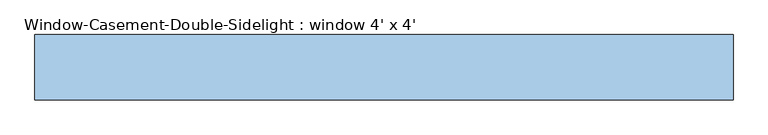
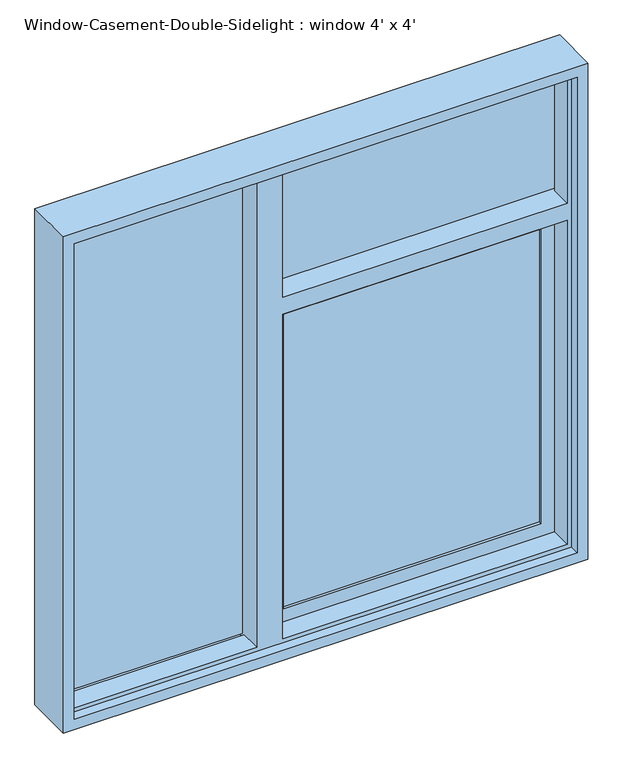
"""IFC4 building model written with IfcOpenShell, lengths in millimetres: window geometry, Window-Casement-Double-Sidelight : window 4' x 4'."""

from ifc_helpers import new_model, si_unit, frame, origin, place, context, project, spatial, polyline, outline, extrude, faceted_brep, source, transform, mapped, element, save


def window_casement_double_sidelight_window_4_x_4_ae1e99d1(model_context):
    return source(origin(), model_context, "Body", "SolidModel", [
        extrude(outline(polyline([(542.3296875, 41.275), (-54.6496875, 41.275), (-54.6496875, 53.975), (542.3296875, 53.975), (542.3296875, 41.275)])), frame((0.0, 0.0, 981.6703125), z_axis=(0.0, 0.0, 1.0), x_axis=(1.0, 0.0, 0.0)), (0.0, 0.0, 1.0), 723.3642187),
        extrude(outline(polyline([(542.3296875, 28.575), (542.3296875, 22.225), (-54.6496875, 22.225), (-54.6496875, 28.575), (542.3296875, 28.575)])), frame((0.0, 0.0, 981.6703125), z_axis=(0.0, 0.0, 1.0), x_axis=(1.0, 0.0, 0.0)), (0.0, 0.0, 1.0), 723.3642187),
        extrude(outline(polyline([(-147.32, 41.275), (-147.32, 34.925), (-584.2, 34.925), (-584.2, 41.275), (-147.32, 41.275)])), frame((0.0, 0.0, 949.9203125), z_axis=(0.0, 0.0, 1.0), x_axis=(1.0, 0.0, 0.0)), (0.0, 0.0, 1.0), 1158.2796875),
        extrude(outline(polyline([(-147.32, 28.575), (-147.32, 22.225), (-584.2, 22.225), (-584.2, 28.575), (-147.32, 28.575)])), frame((0.0, 0.0, 949.9203125), z_axis=(0.0, 0.0, 1.0), x_axis=(1.0, 0.0, 0.0)), (0.0, 0.0, 1.0), 1158.2796875),
        extrude(outline(polyline([(584.2, 28.575), (584.2, 22.225), (-96.52, 22.225), (-96.52, 28.575), (584.2, 28.575)])), frame((0.0, 0.0, 1788.7751563), z_axis=(0.0, 0.0, 1.0), x_axis=(1.0, 0.0, 0.0)), (0.0, 0.0, 1.0), 319.4248438),
        extrude(outline(polyline([(584.2, 41.275), (584.2, 34.925), (-96.52, 34.925), (-96.52, 41.275), (584.2, 41.275)])), frame((0.0, 0.0, 1788.7751563), z_axis=(0.0, 0.0, 1.0), x_axis=(1.0, 0.0, 0.0)), (0.0, 0.0, 1.0), 319.4248438),
        faceted_brep([(-584.2, 15.875, 2108.2), (-584.2, 57.15, 2108.2), (584.2, 57.15, 2108.2), (584.2, 15.875, 2108.2), (-96.52, 15.875, 2108.2), (-96.52, 53.975, 2108.2), (-147.32, 53.975, 2108.2), (-147.32, 15.875, 2108.2), (-574.0796875, -34.925, 2098.0796875), (-574.0796875, 15.875, 2098.0796875), (-147.32, 15.875, 2098.0796875), (-147.32, -34.925, 2098.0796875), (574.0796875, 15.875, 2098.0796875), (574.0796875, -34.925, 2098.0796875), (-86.3996875, -34.925, 2098.0796875), (-86.3996875, 15.875, 2098.0796875), (-584.2, -57.15, 2108.2), (-584.2, -34.925, 2108.2), (584.2, -34.925, 2108.2), (584.2, -57.15, 2108.2), (-609.6, 57.15, 2133.6), (-609.6, -57.15, 2133.6), (609.6, -57.15, 2133.6), (609.6, 57.15, 2133.6), (584.2, 57.15, 939.8), (584.2, 15.875, 939.8), (584.2, 15.875, 1746.9048438), (584.2, 53.975, 1746.9048438), (584.2, 53.975, 1788.7751563), (584.2, 15.875, 1788.7751563), (574.0796875, 15.875, 1788.7751563), (574.0796875, -34.925, 1788.7751563), (574.0796875, 15.875, 949.9203125), (574.0796875, -34.925, 949.9203125), (574.0796875, -34.925, 1746.9048438), (574.0796875, 15.875, 1746.9048438), (584.2, -34.925, 939.8), (584.2, -57.15, 939.8), (609.6, -57.15, 914.4), (609.6, 57.15, 914.4), (-584.2, 57.15, 939.8), (-584.2, 15.875, 939.8), (-147.32, 15.875, 939.8), (-147.32, 53.975, 939.8), (-96.52, 53.975, 939.8), (-96.52, 15.875, 939.8), (-86.3996875, 15.875, 949.9203125), (-86.3996875, -34.925, 949.9203125), (-574.0796875, 15.875, 949.9203125), (-574.0796875, -34.925, 949.9203125), (-147.32, -34.925, 949.9203125), (-147.32, 15.875, 949.9203125), (-584.2, -34.925, 939.8), (-584.2, -57.15, 939.8), (-609.6, -57.15, 914.4), (-609.6, 57.15, 914.4), (-86.3996875, 15.875, 1788.7751563), (-96.52, 15.875, 1788.7751563), (-96.52, 15.875, 1746.9048438), (-86.3996875, 15.875, 1746.9048438), (-86.3996875, -34.925, 1788.7751563), (-86.3996875, -34.925, 1746.9048438), (-96.52, 53.975, 1788.7751563), (-96.52, 53.975, 1746.9048438)], [[[0, 1, 2, 3, 4, 5, 6, 7]], [[8, 9, 10, 11]], [[12, 13, 14, 15]], [[16, 17, 18, 19]], [[20, 21, 22, 23]], [[3, 2, 24, 25, 26, 27, 28, 29]], [[13, 12, 30, 31]], [[32, 33, 34, 35]], [[19, 18, 36, 37]], [[23, 22, 38, 39]], [[25, 24, 40, 41, 42, 43, 44, 45]], [[33, 32, 46, 47]], [[48, 49, 50, 51]], [[37, 36, 52, 53]], [[39, 38, 54, 55]], [[1, 0, 41, 40]], [[12, 15, 56, 57, 4, 3, 29, 30]], [[46, 32, 35, 26, 25, 45, 58, 59]], [[41, 0, 7, 10, 9, 48, 51, 42]], [[9, 8, 49, 48]], [[17, 52, 36, 18], [13, 31, 60, 14], [33, 47, 61, 34], [49, 8, 11, 50]], [[17, 16, 53, 52]], [[22, 21, 54, 38], [16, 19, 37, 53]], [[21, 20, 55, 54]], [[20, 23, 39, 55], [2, 1, 40, 24]], [[43, 6, 5, 62, 28, 27, 63, 44]], [[6, 43, 42, 51, 50, 11, 10, 7]], [[15, 14, 60, 56]], [[47, 46, 59, 61]], [[5, 4, 57, 62]], [[45, 44, 63, 58]], [[63, 27, 26, 35, 34, 61, 59, 58]], [[28, 62, 57, 56, 60, 31, 30, 29]]]),
        extrude(outline(polyline([(1746.9048438, 584.2), (1746.9048438, -96.52), (939.8, -96.52), (939.8, 584.2), (1746.9048438, 584.2)]), holes=[polyline([(981.6703125, 542.3296875), (981.6703125, -54.6496875), (1705.0345313, -54.6496875), (1705.0345313, 542.3296875), (981.6703125, 542.3296875)])]), frame((0.0, 15.875, 0.0), z_axis=(0.0, 1.0, 0.0), x_axis=(0.0, 0.0, 1.0)), (0.0, 0.0, 1.0), 31.75),
    ])


if __name__ == "__main__":
    model = new_model("IFC4")
    model_context = context("Model", 3, world=origin())
    ifc_project = project(units=[si_unit("LENGTHUNIT", "METRE", prefix="MILLI")], contexts=[model_context])
    site = spatial("IfcSite", under=ifc_project)
    building = spatial("IfcBuilding", under=site)
    placement = place(None, origin())
    window_casement_double_sidelight_window_4_x_4_shape = window_casement_double_sidelight_window_4_x_4_ae1e99d1(model_context)
    element("IfcWindow", 1, ObjectType="Window-Casement-Double-Sidelight : window 4' x 4'", at=placement, inside=building, context=model_context, shape_type="MappedRepresentation", body=[
        mapped(window_casement_double_sidelight_window_4_x_4_shape, transform((0.0, 0.0, 0.0), x_axis=(1.0, 0.0, 0.0), y_axis=(0.0, 1.0, 0.0), z_axis=(0.0, 0.0, 1.0))),
    ])
    save(model, "model.ifc")

# Revit data of these elements
# Type "Window-Casement-Double-Sidelight : window 4' x 4'"
#   Type Mark = "22"
#   Fire Rating = "0.5h"
#   Assembly Code = "B2020100"
#   Analytic Construction = "Double glazing - domestic"
#   Window Inset [instance default] = 0' - 0 5/8"
#   Wall Thickness [instance default] = 0' - 6"
#   Visual Light Transmittance = 0.81
#   Transom Height Ratio = 0.3
#   Transom Height = 1' - 2.4"
#   Thermal Resistance (R) = 1.8146 (h·ft²·°F)/BTU
#   Solar Heat Gain Coefficient = 0.76
#   Side Width = 1' - 7.2"
#   Rough Width = 4' - 0 1/2"
#   Rough Height = 4' - 0 1/2"
#   Opening Window Width = 2' - 4.8"
#   Opening Window Height = 2' - 9.6"
#   Heat Transfer Coefficient (U) = 0.5511 BTU/(h·ft²·°F)
#   Height = 4' - 0"
#   Frame Gap 3 [instance default] = 0' - 1 83/128"
#   Frame Gap 2 [instance default] = 0' - 0 5/8"
#   Frame Gap 1 = 0' - 1 51/128"
#   Default Sill Height = 3' - 0"
#   Width = 4' - 0"
#   Frame Material = Metal - Aluminum
#   Glass Panel Material = Glass
#   Wall Closure = (empty or 0)
# Element 1 (IfcWindow, "Window-Casement-Double-Sidelight : window 4' x 4'")
#   Wall Thickness = 0' - 4 1/2"
#   Materials on its faces: "Metal - Aluminum", "Glass"
# Materials
#   "Metal - Aluminum": class "Metal", colour RGB 247 247 247, transparency 0
#   "Glass": class "Glass", colour RGB 0 128 192, transparency 0.75, Description = "Soda Lime Glass", Cost = 0
